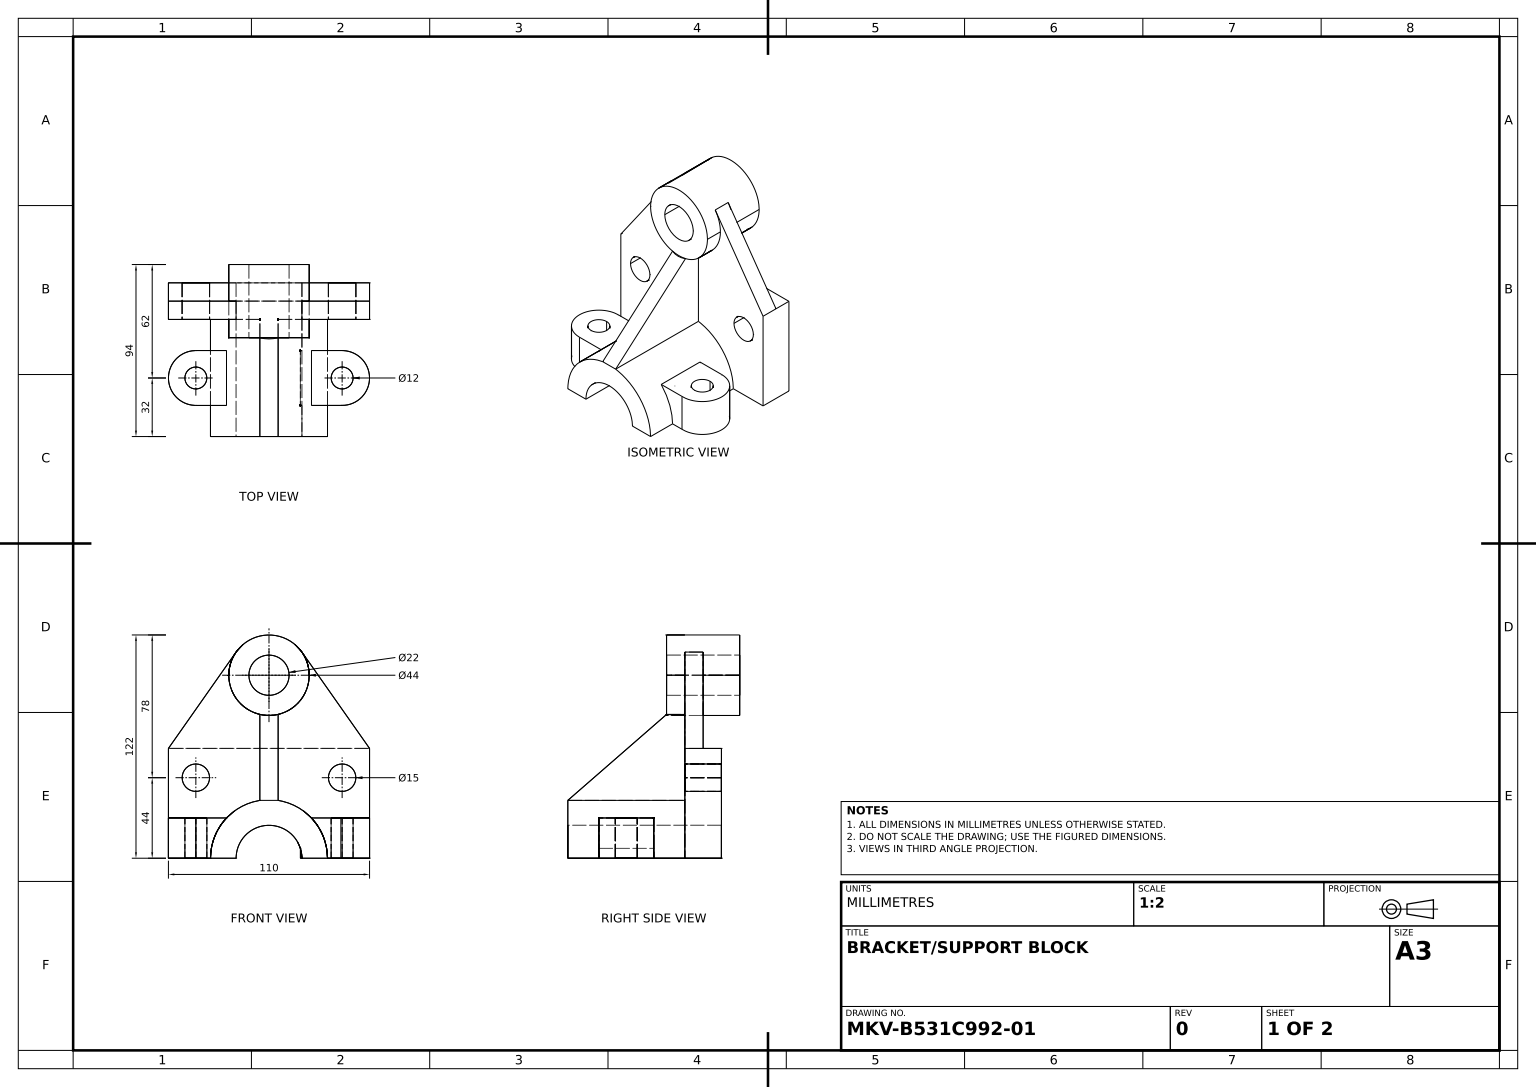
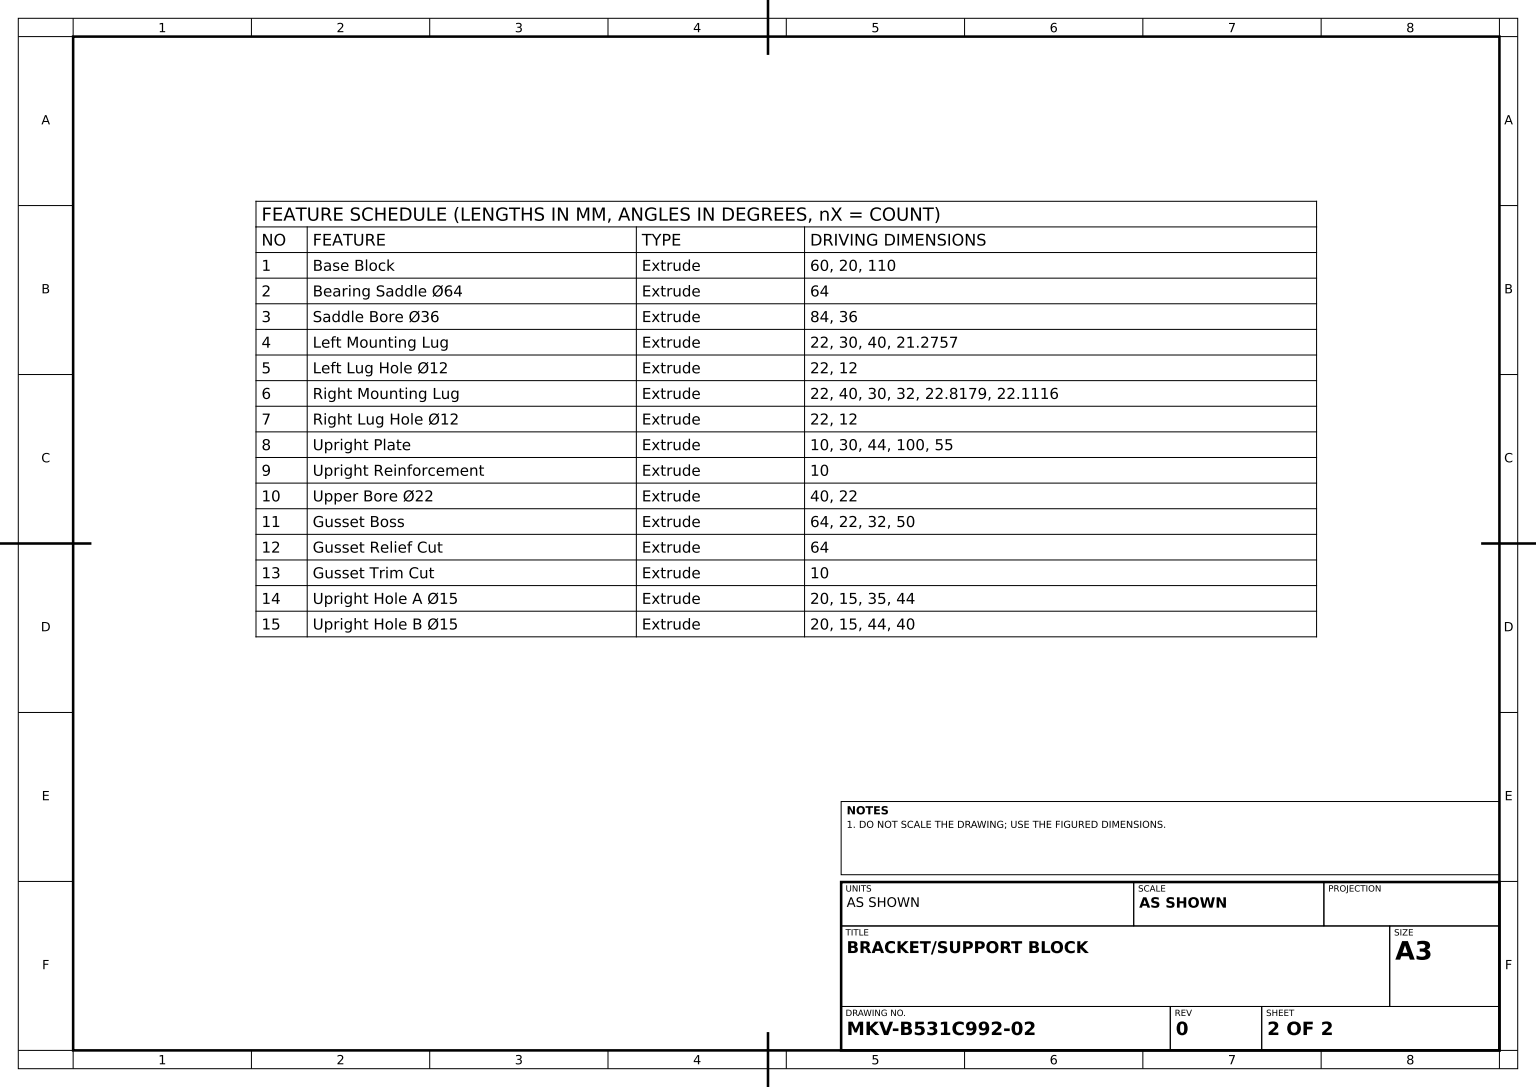
from build123d import *

# Parameters (mm, degrees)
BASE_BLOCK_SKETCH_W         = 110
BASE_BLOCK_SKETCH_H         = 20
BASE_BLOCK_DEPTH            = 60
BEARING_SADDLE_64_DEPTH     = 64
SADDLE_BORE_36_DEPTH        = 84
LEFT_MOUNTING_LUG_DEPTH     = 22
LEFT_LUG_HOLE_SKETCH_R      = 6
LEFT_LUG_HOLE_12_DEPTH      = 22
RIGHT_MOUNTING_LUG_DEPTH    = 22
RIGHT_LUG_HOLE_SKETCH_R     = 6
RIGHT_LUG_HOLE_12_DEPTH     = 22
UPRIGHT_PLATE_DEPTH         = 10
UPRIGHT_PLATE_DEPTH_BACK    = 30
UPRIGHT_PLATE_SKETCH_R      = 22
UPRIGHT_REINFORCEMENT_DEPTH = 10
UPPER_BORE_SKETCH_R         = 11
UPPER_BORE_22_DEPTH         = 40
GUSSET_BOSS_DEPTH           = 64
GUSSET_RELIEF_CUT_DEPTH     = 64
GUSSET_TRIM_CUT_DEPTH       = 10
UPRIGHT_HOLE_A_SKETCH_R     = 7.5
UPRIGHT_HOLE_A_15_DEPTH     = 20
UPRIGHT_HOLE_B_SKETCH_R     = 7.5
UPRIGHT_HOLE_B_15_DEPTH     = 20


with BuildPart() as part:
    # Base Block Sketch → Base Block (new body)
    with BuildSketch(Plane(origin=(0, 0, 0), x_dir=(1, 0, 0), z_dir=(0, 1, 0))):
        with Locations((0, 10)):
            Rectangle(BASE_BLOCK_SKETCH_W, BASE_BLOCK_SKETCH_H)
    extrude(amount=BASE_BLOCK_DEPTH)

    # Bearing Saddle Sketch → Bearing Saddle Ø64 (add)
    with BuildSketch(Plane.XY):
        with BuildLine():
            Line((-32, 0), (32, 0))
            ThreePointArc((32, 0), (0, 32), (-32, 0))
        make_face()
    extrude(amount=BEARING_SADDLE_64_DEPTH)

    # Saddle Bore Sketch → Saddle Bore Ø36 (cut)
    with BuildSketch(Plane.XY.offset(64)):
        with BuildLine():
            Line((-18, 0), (18, 0))
            ThreePointArc((18, 0), (0, 18), (-18, 0))
        make_face()
    extrude(amount=-SADDLE_BORE_36_DEPTH, mode=Mode.SUBTRACT)

    # Left Lug Sketch → Left Mounting Lug (add)
    with BuildSketch(Plane(origin=(0, 0, 0), x_dir=(1, 0, 0), z_dir=(0, 1, 0))):
        with BuildLine():
            Line((-40, -17), (-18.724275485, -17))
            Line((-18.724275485, -17), (-18.724275485, -47))
            Line((-18.724275485, -47), (-40, -47))
            ThreePointArc((-40, -47), (-55, -32), (-40, -17))
        make_face()
    extrude(amount=LEFT_MOUNTING_LUG_DEPTH)

    # Left Lug Hole Sketch → Left Lug Hole Ø12 (cut)
    with BuildSketch(Plane(origin=(0, 22, 0), x_dir=(1, 0, 0), z_dir=(0, 1, 0))):
        with Locations(Location((-40, -32, 0), (0, 0, 270))):
            Circle(LEFT_LUG_HOLE_SKETCH_R)
    extrude(amount=-LEFT_LUG_HOLE_12_DEPTH, mode=Mode.SUBTRACT)

    # Right Lug Sketch → Right Mounting Lug (add)
    with BuildSketch(Plane(origin=(0, 0, 0), x_dir=(1, 0, 0), z_dir=(0, 1, 0))):
        with BuildLine():
            Line((40, -17), (17.182133471, -17))
            Line((17.182133471, -17), (17.182133471, -47))
            Line((17.182133471, -47), (39.293701119, -46.983362169))
            ThreePointArc((39.293701119, -46.983362169), (54.995839965, -32.353247409), (40, -17))
        make_face()
    extrude(amount=RIGHT_MOUNTING_LUG_DEPTH)

    # Right Lug Hole Sketch → Right Lug Hole Ø12 (cut)
    with BuildSketch(Plane(origin=(0, 22, 0), x_dir=(1, 0, 0), z_dir=(0, 1, 0))):
        with Locations(Location((40, -32, 0), (0, 0, 270))):
            Circle(RIGHT_LUG_HOLE_SKETCH_R)
    extrude(amount=-RIGHT_LUG_HOLE_12_DEPTH, mode=Mode.SUBTRACT)



with BuildPart() as body_2:
    # Upright Plate Sketch → Upright Plate (new, two sides: drawn at the far end of the back side and taken through both)
    with BuildSketch(Plane.XY.offset(-UPRIGHT_PLATE_DEPTH_BACK)):
        with Locations((0, 100)):
            Circle(UPRIGHT_PLATE_SKETCH_R)
    extrude(amount=UPRIGHT_PLATE_DEPTH + UPRIGHT_PLATE_DEPTH_BACK)


with BuildPart() as part_1:
    add(part.part)

    add(body_2.part)  # Upright Reinforcement merges body 2
    # Upright Reinforcement Sketch → Upright Reinforcement (add)
    with BuildSketch(Plane.XY):
        with BuildLine():
            Line((-55, 60), (-17.999682143, 112.649562947))
            ThreePointArc((-17.999682143, 112.649562947), (0, 78), (17.999682143, 112.649562947))
            Line((17.999682143, 112.649562947), (55, 60))
            Line((55, 60), (-55, 60))
        make_face()
    extrude(amount=-UPRIGHT_REINFORCEMENT_DEPTH)

    # Upper Bore Sketch → Upper Bore Ø22 (cut)
    with BuildSketch(Plane.XY.offset(10)):
        with Locations((0, 100)):
            Circle(UPPER_BORE_SKETCH_R)
    extrude(amount=-UPPER_BORE_22_DEPTH, mode=Mode.SUBTRACT)

    # Gusset Boss Sketch → Gusset Boss (add)
    with BuildSketch(Plane.XY):
        with BuildLine():
            Line((-5, 78.575714714), (-5, 31.606961259))
            ThreePointArc((-5, 31.606961259), (0, 32), (5, 31.606961259))
            Line((5, 31.606961259), (5, 78.575714714))
            ThreePointArc((5, 78.575714714), (0, 78), (-5, 78.575714714))
        make_face()
    extrude(amount=GUSSET_BOSS_DEPTH)

    # Gusset Relief Sketch → Gusset Relief Cut (cut)
    with BuildSketch(Plane(origin=(0, 0, 0), x_dir=(0, 0, -1), z_dir=(1, 0, 0))):
        Polygon((-10, 78.575714714), (-64, 31.606961259), (-64, 78.575714714), align=None)
    extrude(amount=-GUSSET_RELIEF_CUT_DEPTH, mode=Mode.SUBTRACT)

    # Gusset Trim Sketch → Gusset Trim Cut (cut)
    with BuildSketch(Plane.ZY):
        Polygon((10, 78.575714714), (64, 31.606961259), (64, 78.575714714), align=None)
    extrude(amount=-GUSSET_TRIM_CUT_DEPTH, mode=Mode.SUBTRACT)

    # Upright Hole A Sketch → Upright Hole A Ø15 (cut)
    with BuildSketch(Plane.XY):
        with Locations((40, 44)):
            Circle(UPRIGHT_HOLE_A_SKETCH_R)
    extrude(amount=-UPRIGHT_HOLE_A_15_DEPTH, mode=Mode.SUBTRACT)

    # Upright Hole B Sketch → Upright Hole B Ø15 (cut)
    with BuildSketch(Plane.XY):
        with Locations((-40, 44)):
            Circle(UPRIGHT_HOLE_B_SKETCH_R)
    extrude(amount=-UPRIGHT_HOLE_B_15_DEPTH, mode=Mode.SUBTRACT)


solid = part_1.part
